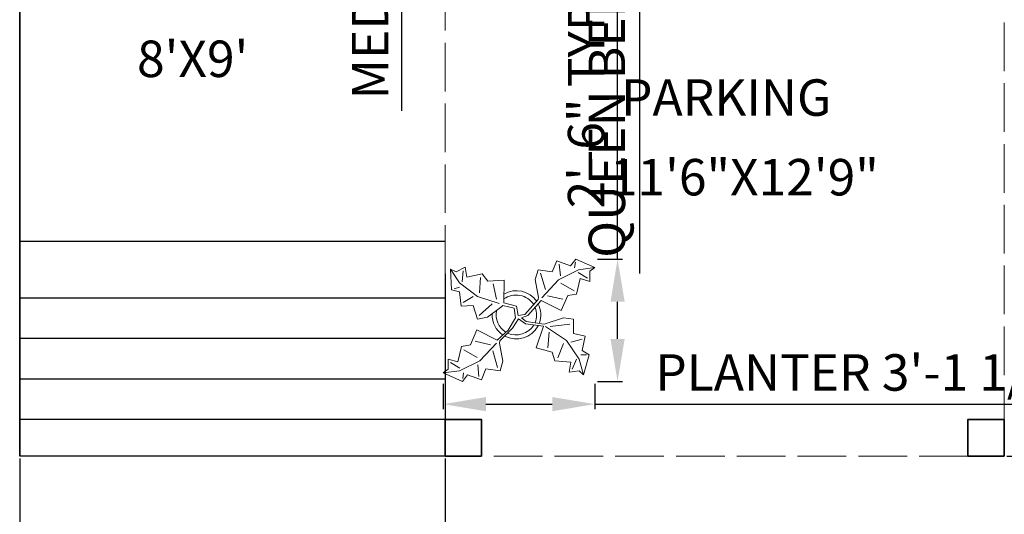
# Model space of a CAD drawing. Units: inches. Extents: x 1956 to 4770, y 1551 to 2596.
# Tile 2 of 10: x 2258 to 2501, y 1743 to 1865. Entities that reach past the tile are written whole.
import ezdxf

# ---------------------------------------------------------------- set-up
doc = ezdxf.new("R2010")
doc.units = ezdxf.units.IN
doc.linetypes.add('ACAD_ISO02W100', pattern=[15, 12, -3])
for name, color, linetype, lineweight in [('A-ANNO-DIMS', 2, 'Continuous', 18), ('A-AREA-IDEN', 7, 'Continuous', 18), ('A-FLOR-OVHD', 8, 'ACAD_ISO02W100', 18), ('A-FLOR-STRS', 7, 'Continuous', 25), ('A-WALL', 7, 'Continuous', 35), ('L-PLNT', 116, 'Continuous', 18), ('S-COLS', 5, 'Continuous', 35)]:
    doc.layers.add(name, color=color, linetype=linetype, lineweight=lineweight)
doc.styles.get("Standard").update_dxf_attribs({"font": 'arial.ttf'})
doc.dimstyles.new('ISO-25', dxfattribs={"dimtxt": 9, "dimasz": 10.5, "dimexe": 1.25, "dimexo": 0.625, "dimgap": 2, "dimtad": 1, "dimdec": 1, "dimlunit": 4, "dimtxsty": 'Standard', "dimcen": 2.5, "dimadec": 0, "dimazin": 0, "dimtfac": 1, "dimtdec": 1, "dimtmove": 0, "dimatfit": 3, "dimfxl": 1, "dimarcsym": 0})

# ---------------------------------------------------------------- blocks, each defined once
blk = doc.blocks.new('*D1')
at = {"layer": 'A-ANNO-DIMS', "color": 0, "lineweight": -2, "transparency": 16777216}
for p, q in [((2501.88, 2309.09), (2599.11, 2309.09)), ((2597.86, 2298.59), (2597.86, 1767.59)), ((2501.88, 1757.09), (2599.11, 1757.09))]:
    blk.add_line(p, q, dxfattribs=at)
at = {"layer": 'A-ANNO-DIMS', "color": 0, "transparency": 16777216}
for points in [[(2596.11, 2298.59), (2599.61, 2298.59), (2597.86, 2309.09)], [(2596.11, 1767.59), (2599.61, 1767.59), (2597.86, 1757.09)]]:
    blk.add_solid(points, dxfattribs=at)
at = {"layer": 'Defpoints', "color": 0, "transparency": 16777216}
for p in [(2501.25, 2309.09), (2501.25, 1757.09), (2597.86, 1757.09)]:
    blk.add_point(p, dxfattribs=at)
at = {"layer": 'A-ANNO-DIMS', "color": 0, "transparency": 16777216, "insert": (2591.27, 2033.09), "char_height": 9, "attachment_point": 5, "rotation": 90}
blk.add_mtext("46'", dxfattribs=at)
blk = doc.blocks.new('Plant - Rubber or Philodendron')
for p, q in [((8.8871, 10.7908), (9.9809, 13.4933)), ((9.9809, 13.4933), (13.3837, 12.301)), ((10.5828, 12.6946), (10.8893, 9.7953)), ((13.3837, 12.301), (14.68, 13.9039)), ((14.5816, 13.2037), (14.3848, 11.8033)), ((14.68, 13.9039), (19.3848, 11.8146)), ((-16.2005, 11.4774), (-13.9899, 8.1064)), ((-16.2005, 11.4774), (-14.8639, 10.7964)), ((-16.0159, 6.3329), (-16.2005, 11.4774)), ((-14.8639, 10.7964), (-12.6195, 11.8975)), ((-13.3174, 8.325), (-13.0735, 11.0065)), ((-12.6195, 11.8975), (-12.1909, 9.4345)), ((-12.1909, 9.4345), (-8.3829, 10.3)), ((-8.3829, 10.3), (-7.0549, 8.501)), ((4.6914, 8.8812), (5.3859, 11.2828)), ((5.3859, 11.2828), (8.8871, 10.7908)), ((5.9878, 10.4842), (7.1971, 6.3869)), ((15.3859, 11.3055), (10.3916, 8.7942)), ((15.2875, 10.6053), (17.5907, 9.2105)), ((19.3848, 11.8146), (15.3859, 11.3055)), ((19.3848, 11.8146), (18.1868, 10.9119)), ((18.1868, 10.9119), (18.1925, 8.4119)), ((-13.9899, 8.1064), (-9.5434, 4.7185)), ((-8.8369, 9.409), (-9.0894, 5.6095)), ((-7.0549, 8.501), (-3.0284, 8.6941)), ((-4.8529, 4.012), (-5.7184, 7.82)), ((-3.0284, 8.6941), (-3.0709, 3.1041)), ((4.6914, 8.8812), (5.5014, 4.4831)), ((10.3916, 8.7942), (6.2847, 4.4028)), ((14.2977, 6.1031), (10.9934, 7.9956)), ((15.7909, 9.1065), (14.8995, 5.3044)), ((18.1925, 8.4119), (15.7909, 9.1065)), ((-14.0069, 5.8704), (-16.0159, 6.3329)), ((-15.3434, 6.5514), (-13.9984, 6.9884)), ((-13.5868, 2.2894), (-14.0069, 5.8704)), ((7.7005, 4.8881), (11.5025, 3.9967)), ((12.7005, 4.8994), (11.1089, 1.1958)), ((14.8995, 5.3044), (12.7005, 4.8994)), ((-10.6784, 2.491), (-13.5868, 2.2894)), ((-13.1329, 3.1804), (-10.6614, 4.727)), ((-9.5858, -0.8715), (-10.6784, 2.491)), ((-9.5434, 4.7185), (-4.1917, 2.9888)), ((-9.1318, 0.0195), (-5.9793, 2.9025)), ((-3.5248, 2.2131), (-3.3011, 2.4355)), ((-3.3011, 2.4355), (-0.5306, 1.7947)), ((-3.0709, 3.1041), (0.0797, 2.3163)), ((2.1141, 0.2298), (5.4346, 3.9146)), ((6.1032, 3.6844), (2.8262, -0.031)), ((5.4346, 3.9146), (5.5014, 4.4831)), ((11.1089, 1.1958), (6.1032, 3.6844)), ((-7.1228, -0.443), (-3.5248, 2.2131)), ((-0.5306, 1.7947), (-0.2255, -0.5527)), ((-0.5306, 1.7947), (-0.5306, 1.7947)), ((0.0797, 2.3163), (0.4866, -0.031)), ((0.4866, -0.031), (2.1141, 0.2298)), ((-7.1228, -0.443), (-9.5858, -0.8715)), ((-2.019, -3.6148), (-0.2255, -0.5527)), ((-0.9375, -3.1608), (0.5883, -0.8135)), ((0.5883, -0.8135), (2.2447, -2.0916)), ((2.8262, -0.031), (1.3003, -0.5527)), ((1.3003, -0.5527), (2.4193, -1.4655)), ((2.2447, -2.0916), (6.7108, -2.6626)), ((2.4193, -1.4655), (6.895, -2.1175)), ((11.6605, -0.5413), (6.895, -2.1175)), ((8.3544, -2.7453), (13.1973, -2.1704)), ((11.6605, -0.5413), (14.1354, -0.8948)), ((14.1354, -0.8948), (14.1354, -4.4304)), ((-11.3237, -7.2629), (-9.7321, -3.5593)), ((-9.7321, -3.5593), (-4.7264, -6.0479)), ((-2.019, -3.6148), (-4.7264, -6.0479)), ((-4.0579, -6.2781), (-0.9375, -3.1608)), ((4.943, -7.9659), (6.7108, -2.6626)), ((12.3677, -6.1981), (7.219, -2.6772)), ((8.125, -4.0768), (7.7715, -7.9659)), ((14.1354, -4.4304), (16.9638, -5.1375)), ((-13.5228, -7.6679), (-11.3237, -7.2629)), ((-6.3237, -7.2516), (-10.1257, -6.3602)), ((-9.0148, -11.1577), (-4.9047, -6.8122)), ((-4.1246, -6.8466), (-4.0579, -6.2781)), ((-3.3146, -11.2447), (-4.1246, -6.8466)), ((10.2463, -10.4408), (11.6605, -6.9053)), ((15.5496, -10.7943), (12.3677, -6.1981)), ((16.2567, -5.8446), (13.4283, -6.5517)), ((16.9638, -5.1375), (16.2567, -8.673)), ((-14.4141, -11.4699), (-13.5228, -7.6679)), ((-12.921, -8.4665), (-9.6166, -10.359)), ((-4.611, -12.8477), (-5.8203, -8.7504)), ((8.8321, -9.0266), (4.943, -7.9659)), ((9.5392, -11.1479), (8.8321, -9.0266)), ((16.2567, -8.673), (18.0245, -9.7337)), ((-16.8157, -10.7754), (-14.4141, -11.4699)), ((-16.8101, -13.2754), (-16.8157, -10.7754)), ((-13.9107, -12.9688), (-16.2139, -11.574)), ((-14.0091, -13.669), (-9.0148, -11.1577)), ((-3.3146, -11.2447), (-4.0092, -13.6463)), ((13.4283, -11.5015), (9.5392, -11.1479)), ((13.0748, -13.9763), (13.4283, -11.5015)), ((14.8425, -10.7943), (13.7819, -13.2692)), ((16.6103, -14.6834), (15.5496, -10.7943)), ((17.3174, -9.7337), (15.9032, -9.7337)), ((18.0245, -9.7337), (16.6103, -14.6834)), ((-18.008, -14.1781), (-16.8101, -13.2754)), ((-18.008, -14.1781), (-14.0091, -13.669)), ((-13.3032, -16.2674), (-18.008, -14.1781)), ((-13.2048, -15.5672), (-13.008, -14.1668)), ((-9.206, -15.0581), (-9.5126, -12.1588)), ((-7.5103, -13.1543), (-8.6042, -15.8568)), ((-4.0092, -13.6463), (-7.5103, -13.1543)), ((15.5496, -13.6228), (13.0748, -13.9763)), ((16.6103, -14.6834), (15.5496, -13.6228)), ((-12.0069, -14.6645), (-13.3032, -16.2674)), ((-8.6042, -15.8568), (-12.0069, -14.6645))]:
    blk.add_line(p, q)
for centre, radius, start, end in [((0, 0), 6.1275, 34.37569, 120.1028), ((-0.0601, -0.2075), 5.2461, 33.82192, 124.9414), ((-0.098, 0.1364), 6.1288, 341.2017, 26.09184), ((0.0308, 0.1664), 6, 178.6147, 235.1169), ((0.0308, 0.1664), 5, 168.1647, 238.6725), ((-0.2664, 0.1682), 5.2775, 338.4094, 20.03007), ((-0.1102, 0.4886), 5.2883, 247.3711, 327.472), ((-0.0234, 0.3825), 6.1492, 242.5812, 331.2714)]:
    blk.add_arc(centre, radius, start, end)
blk = doc.blocks.new('COL-PORCH-9X9')
blk.add_line((0, 0), (9, 0))
blk.add_lwpolyline([(0, 0), (0, 9), (9, 9), (9, 0)])
blk = doc.blocks.new('*D39')
at = {"layer": 'A-ANNO-DIMS', "color": 0, "lineweight": -2, "transparency": 16777216}
for p, q in [((2362.8, 1774.88), (2362.8, 1768.65)), ((2400.2, 1774.88), (2400.2, 1768.65)), ((2373.3, 1769.9), (2389.7, 1769.9)), ((2400.2, 1769.9), (2551.56, 1769.9))]:
    blk.add_line(p, q, dxfattribs=at)
at = {"layer": 'A-ANNO-DIMS', "color": 0, "transparency": 16777216}
for points in [[(2373.3, 1771.65), (2373.3, 1768.15), (2362.8, 1769.9)], [(2389.7, 1771.65), (2389.7, 1768.15), (2400.2, 1769.9)]]:
    blk.add_solid(points, dxfattribs=at)
at = {"layer": 'Defpoints', "color": 0, "transparency": 16777216}
for p in [(2362.8, 1775.51), (2400.2, 1775.51), (2400.2, 1769.9)]:
    blk.add_point(p, dxfattribs=at)
at = {"layer": 'A-ANNO-DIMS', "color": 0, "transparency": 16777216, "insert": (2481.13, 1776.56), "char_height": 9, "attachment_point": 5}
blk.add_mtext('PLANTER 3\'-1 1/2" TYP.', dxfattribs=at)
blk = doc.blocks.new('*D40')
at = {"layer": 'A-ANNO-DIMS', "color": 0, "lineweight": -2, "transparency": 16777216}
for p, q in [((2405.81, 1805.68), (2405.81, 1875.19)), ((2400.82, 1805.68), (2407.06, 1805.68)), ((2405.81, 1786.01), (2405.81, 1795.18)), ((2400.82, 1775.51), (2407.06, 1775.51))]:
    blk.add_line(p, q, dxfattribs=at)
at = {"layer": 'A-ANNO-DIMS', "color": 0, "transparency": 16777216}
for points in [[(2404.06, 1795.18), (2407.56, 1795.18), (2405.81, 1805.68)], [(2404.06, 1786.01), (2407.56, 1786.01), (2405.81, 1775.51)]]:
    blk.add_solid(points, dxfattribs=at)
at = {"layer": 'Defpoints', "color": 0, "transparency": 16777216}
for p in [(2400.2, 1805.68), (2405.81, 1805.68), (2400.2, 1775.51)]:
    blk.add_point(p, dxfattribs=at)
at = {"layer": 'A-ANNO-DIMS', "color": 0, "transparency": 16777216, "insert": (2399.21, 1845.69), "char_height": 9, "attachment_point": 5, "rotation": 90}
blk.add_mtext('2\'-6" TYP.', dxfattribs=at)
blk = doc.blocks.new('*D45')
at = {"layer": 'A-ANNO-DIMS', "color": 0, "lineweight": -2, "transparency": 16777216}
for p, q in [((2422.63, 1998.09), (2410, 1998.09)), ((2411.25, 1987.59), (2411.25, 1928.59)), ((2422.63, 1918.09), (2410, 1918.09)), ((2411.25, 1918.09), (2411.25, 1802.13))]:
    blk.add_line(p, q, dxfattribs=at)
at = {"layer": 'A-ANNO-DIMS', "color": 0, "transparency": 16777216}
for points in [[(2409.5, 1987.59), (2413, 1987.59), (2411.25, 1998.09)], [(2409.5, 1928.59), (2413, 1928.59), (2411.25, 1918.09)]]:
    blk.add_solid(points, dxfattribs=at)
at = {"layer": 'Defpoints', "color": 0, "transparency": 16777216}
for p in [(2423.25, 1998.09), (2411.25, 1918.09), (2423.25, 1918.09)]:
    blk.add_point(p, dxfattribs=at)
at = {"layer": 'A-ANNO-DIMS', "color": 0, "transparency": 16777216, "insert": (2404.32, 1854.86), "char_height": 9, "attachment_point": 5, "rotation": 90}
blk.add_mtext('QUEEN BED 6\'-8"', dxfattribs=at)
blk = doc.blocks.new('*D61')
at = {"layer": 'A-ANNO-DIMS', "color": 0, "lineweight": -2, "transparency": 16777216}
for p, q in [((2359.65, 2008.45), (2351.23, 2008.45)), ((2352.48, 1997.95), (2352.48, 1966.95)), ((2359.65, 1956.45), (2351.23, 1956.45)), ((2352.48, 1956.45), (2352.48, 1842.3))]:
    blk.add_line(p, q, dxfattribs=at)
at = {"layer": 'A-ANNO-DIMS', "color": 0, "transparency": 16777216}
for points in [[(2350.73, 1997.95), (2354.23, 1997.95), (2352.48, 2008.45)], [(2350.73, 1966.95), (2354.23, 1966.95), (2352.48, 1956.45)]]:
    blk.add_solid(points, dxfattribs=at)
at = {"layer": 'Defpoints', "color": 0, "transparency": 16777216}
for p in [(2360.28, 2008.45), (2352.48, 1956.45), (2360.28, 1956.45)]:
    blk.add_point(p, dxfattribs=at)
at = {"layer": 'A-ANNO-DIMS', "color": 0, "transparency": 16777216, "insert": (2345.9, 1894.13), "char_height": 9, "attachment_point": 5, "rotation": 90}
blk.add_mtext('MEDIA UNIT 4\'-4"', dxfattribs=at)
blk = doc.blocks.new('*D63')
at = {"layer": 'A-ANNO-DIMS', "color": 0, "lineweight": -2, "transparency": 16777216}
for p, q in [((2258.25, 1756.46), (2258.25, 1721.79)), ((2363.25, 1756.46), (2363.25, 1721.79)), ((2268.75, 1723.04), (2352.75, 1723.04))]:
    blk.add_line(p, q, dxfattribs=at)
at = {"layer": 'A-ANNO-DIMS', "color": 0, "transparency": 16777216}
for points in [[(2268.75, 1724.79), (2268.75, 1721.29), (2258.25, 1723.04)], [(2352.75, 1724.79), (2352.75, 1721.29), (2363.25, 1723.04)]]:
    blk.add_solid(points, dxfattribs=at)
at = {"layer": 'Defpoints', "color": 0, "transparency": 16777216}
for p in [(2258.25, 1757.09), (2363.25, 1757.09), (2363.25, 1723.04)]:
    blk.add_point(p, dxfattribs=at)
at = {"layer": 'A-ANNO-DIMS', "color": 0, "transparency": 16777216, "insert": (2310.75, 1729.63), "char_height": 9, "attachment_point": 5}
blk.add_mtext('8\'-9"', dxfattribs=at)

msp = doc.modelspace()

# ---------------------------------------------------------------- linework, layer by layer
at = {"layer": 'A-FLOR-OVHD'}
for p, q in [((2363.25, 1802.09), (2363.25, 1918.09)), ((2501.25, 1909.09), (2501.25, 1757.09)), ((2363.25, 1757.09), (2363.25, 1766.09)), ((2492.25, 1757.09), (2372.25, 1757.09))]:
    msp.add_line(p, q, dxfattribs=at)
at = {"layer": 'A-FLOR-STRS'}
for p, q in [((2258.25, 1810.09), (2363.25, 1810.09)), ((2363.25, 1802.09), (2363.25, 1757.09)), ((2363.25, 1796.09), (2258.25, 1796.09)), ((2363.25, 1786.09), (2258.25, 1786.09)), ((2363.25, 1776.09), (2258.25, 1776.09)), ((2363.25, 1766.09), (2258.25, 1766.09)), ((2363.25, 1757.09), (2258.25, 1757.09))]:
    msp.add_line(p, q, dxfattribs=at)
at = {"layer": 'A-WALL'}
msp.add_line((2258.25, 1757.09), (2258.25, 2309.09), dxfattribs=at)

# ---------------------------------------------------------------- block references
at = {"layer": 'L-PLNT'}
msp.add_blockref('Plant - Rubber or Philodendron', (2380.81, 1791.78), dxfattribs=at)
at = {"layer": 'S-COLS'}
for p in [(2363.25, 1757.09), (2492.25, 1757.09)]:
    msp.add_blockref('COL-PORCH-9X9', p, dxfattribs=at)

# ---------------------------------------------------------------- texts
at = {"layer": 'A-AREA-IDEN'}
for s, p in [("    8'X9'", (2276.21, 1850.64)), (' PARKING ', (2403.9, 1841.07)), ('11\'6"X12\'9"', (2403.9, 1821.42))]:
    msp.add_text(s, height=9, dxfattribs=at).set_placement(p)

# ---------------------------------------------------------------- dimensions: what is measured, and where the dimension line sits
at = {"layer": 'A-ANNO-DIMS'}
dim = msp.add_linear_dim(base=(2597.86, 1757.09), p1=(2501.25, 2309.09), p2=(2501.25, 1757.09), angle=90, dimstyle='ISO-25', override={"dimclrd": 0, "dimclre": 0, "dimclrt": 0}, dxfattribs=at)
dim.commit()
dim.dimension.update_dxf_attribs({"geometry": '*D1', "text_midpoint": (2591.27, 2033.09)})
for base, p1, p2, angle, text, picture, middle in [((2352.48, 1956.45), (2360.28, 2008.45), (2360.28, 1956.45), 270, 'MEDIA UNIT <>', '*D61', (2345.9, 1894.13)), ((2411.25, 1918.09), (2423.25, 1998.09), (2423.25, 1918.09), 270, 'QUEEN BED <>', '*D45', (2404.32, 1854.86)), ((2405.81, 1805.68), (2400.2, 1775.51), (2400.2, 1805.68), 90, '<> TYP.', '*D40', (2399.21, 1845.69))]:
    dim = msp.add_linear_dim(base=base, p1=p1, p2=p2, angle=angle, text=text, dimstyle='ISO-25', override={"dimdec": 1, "dimlfac": 1, "dimrnd": 0, "dimzin": 1, "dimdsep": 46, "dimlunit": 4, "dimfrac": 2}, dxfattribs=at)
    dim.commit()
    dim.dimension.update_dxf_attribs({"geometry": picture, "text_midpoint": middle})
dim = msp.add_linear_dim(base=(2400.2, 1769.9), p1=(2362.8, 1775.51), p2=(2400.2, 1775.51), text='PLANTER <> TYP.', dimstyle='ISO-25', override={"dimdec": 1, "dimlfac": 1, "dimrnd": 0, "dimzin": 1, "dimdsep": 46, "dimlunit": 4, "dimfrac": 2}, dxfattribs=at)
dim.commit()
dim.dimension.update_dxf_attribs({"geometry": '*D39', "text_midpoint": (2481.13, 1776.56)})
dim = msp.add_linear_dim(base=(2363.25, 1723.04), p1=(2258.25, 1757.09), p2=(2363.25, 1757.09), dimstyle='ISO-25', override={"dimdec": 1, "dimlfac": 1, "dimrnd": 0, "dimzin": 1, "dimdsep": 46, "dimlunit": 4, "dimfrac": 2}, dxfattribs=at)
dim.commit()
dim.dimension.update_dxf_attribs({"geometry": '*D63', "text_midpoint": (2310.75, 1729.63)})

doc.saveas('drawing.dxf')
